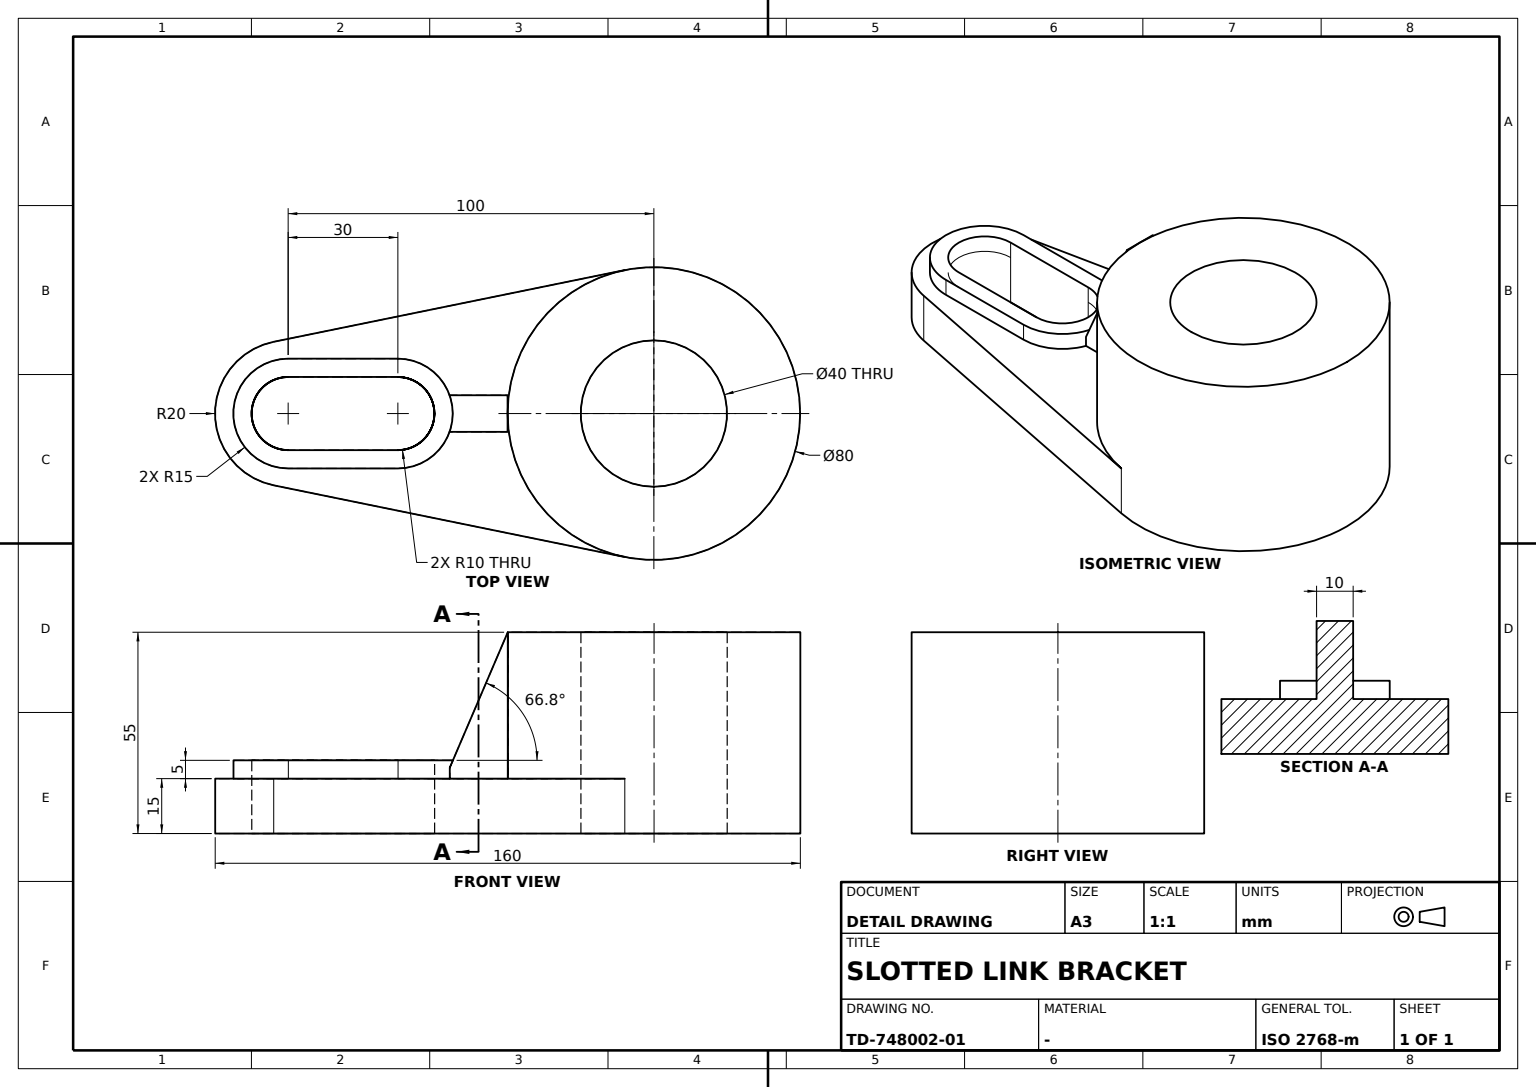
CATIA V5 part; units mm, degrees
sketch "Sketch1" plane through (0, 0, 0) normal (0, 0, 1) x (0, 1, 0)
  circle A0 centre (0, 0) radius 40
  dimension "radius A0" = 40
extrude "Pad1" add sketch "Sketch1" along normal blind 55
sketch "Sketch2" plane through (0, 0, 55) normal (0, 0, 1) x (1, 0, 0)
  circle A0 centre (0, 0) radius 20
  point P0 (0, 0)
  circle A1 centre (0, 0) radius 40 construction
  dimension "radius A0" = 20
  constraint coincidence P0 y-axis
  constraint concentricity A0 A1
extrude "Pocket1" cut sketch "Sketch2" against normal through all
sketch "Sketch3" plane through (0, 0, 0) normal (0, 0, 1) x (0, 1, 0)
  line L0 (-100, 0) -> (-70, 0) construction
  point P0 (-100, 0)
  line L1 (-100, 10) -> (-70, 10)
  line L2 (-70, -10) -> (-100, -10)
  arc A0 (-70, 10) -> (-70, -10) centre (-70, 0) cw
  arc A1 (-100, -10) -> (-100, 10) centre (-100, 0) cw
  line L3 (-100, 0) -> (-70, 0) construction
  line L4 (-100, 15) -> (-70, 15)
  line L5 (-70, -15) -> (-100, -15)
  arc A2 (-70, 15) -> (-70, -15) centre (-70, 0) cw
  arc A3 (-100, -15) -> (-100, 15) centre (-100, 0) cw
  dimension "length L0" = 30
  dimension "distance L0 L1" = 10
  dimension "distance L3 L4" = 15
  dimension "distance P0 origin" = 100
  constraint coincidence P0 x-axis
  constraint horizontal L0 x-axis
  constraint horizontal L3 x-axis
  constraint tangency A0 L1
  constraint tangency A1 L1
  constraint tangency A0 L2
  constraint tangency A1 L2
  constraint tangency A2 L4
  constraint tangency A3 L4
  constraint tangency A2 L5
  constraint tangency A3 L5
extrude "Pad2" add sketch "Sketch3" along normal blind 20
sketch "Sketch4" plane through (0, 0, 0) normal (0, 0, 1) x (0, 1, 0)
  circle A0 centre (0, 0) radius 40 construction
  arc A1 (-8, 39.1918) -> (-8, -39.1918) centre (0, 0) ccw
  arc A2 (-104, 19.5959) -> (-104, -19.5959) centre (-100, 0) ccw
  point P0 (-100, 0)
  arc A3 (-100, 15) -> (-100, -15) centre (-100, 0) ccw construction
  line L0 (-104, 19.5959) -> (-8, 39.1918)
  point P1 (-8, 39.1918)
  line L1 (-104, -19.5959) -> (-8, -39.1918)
  point P2 (-8, -39.1918)
  dimension "radius A2" = 20
  constraint coincidence P0 x-axis
  constraint coincidence A0 P1
  constraint coincidence A0 P2
  constraint concentricity A2 A3
  constraint tangency L0 A2
  constraint tangency L0 A0
  constraint tangency L1 A2
  constraint tangency L1 A0
extrude "Pad3" add sketch "Sketch4" along normal blind 15
sketch "Sketch5" plane through (0, 0, 0) normal (1, 0, 0) x (0, 1, 0)
  point P0 (-55, 20)
  point P1 (-55, 20)
  line L0 (-40, 55) -> (-40, 15)
  line L1 (-40, 55) -> (-55, 20)
  point P2 (-55, 20)
  constraint vertical L0 y-axis
  constraint coincidence P0 P2
rib "Stiffener1" sketch "Sketch5" thickness 10 sides both
sketch "Sketch6" plane through (0, 0, 15) normal (0, 0, 1) x (1, 0, 0)
  line L0 (10, -100) -> (10, -70)
  arc A0 (-10, -70) -> (10, -70) centre (0, -70) cw
  line L1 (-10, -70) -> (-10, -100)
  arc A1 (10, -100) -> (-10, -100) centre (0, -100) cw
extrude "Pocket2" cut sketch "Sketch6" against normal through all
properties part number "2D Engineering Drawing of a Slotted Link Bracket with Circular Mounting Boss in CATIA"
